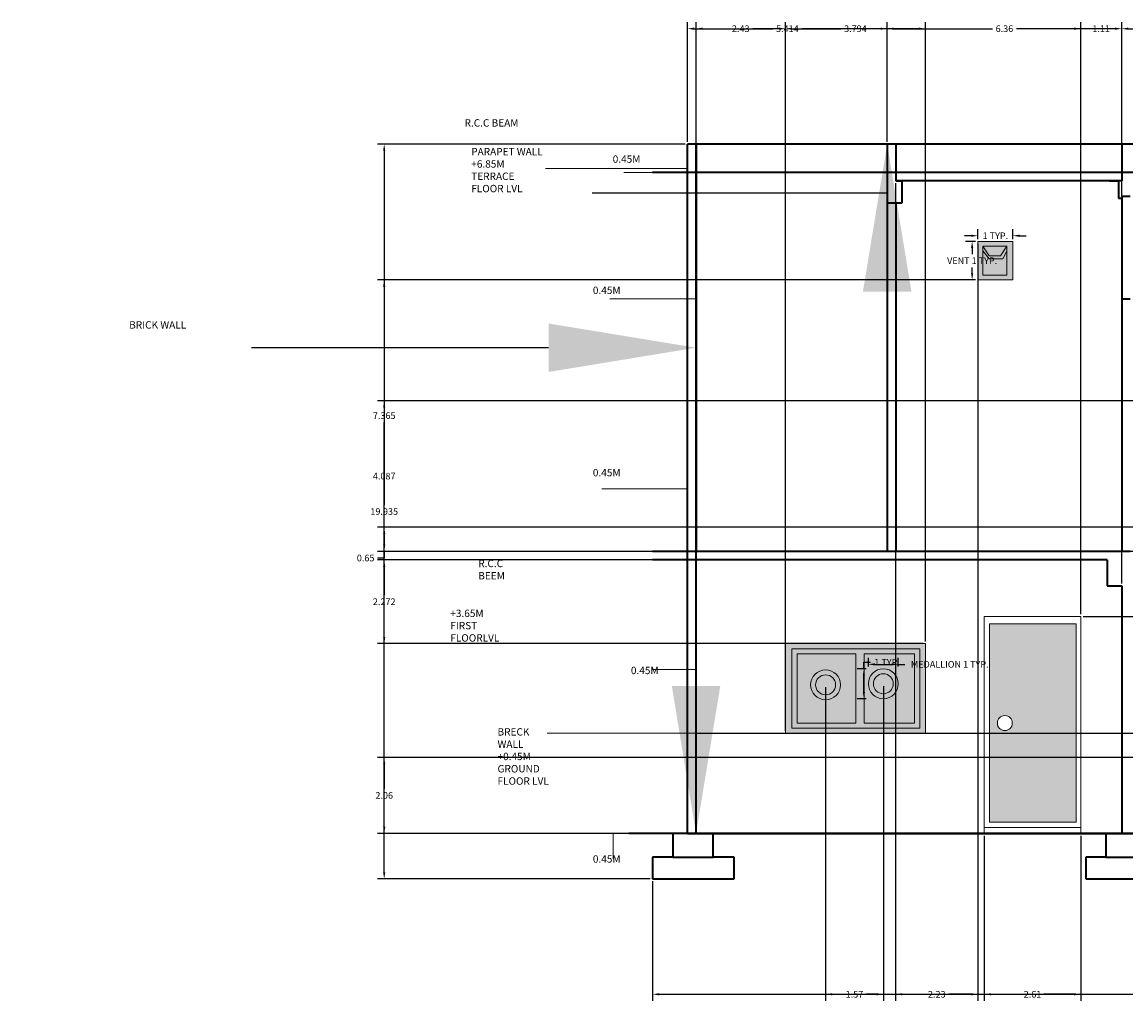
# Model space of a CAD drawing. Units: metres. Extents: x 1976.6 to 2045, y 823.7 to 850.3.
# Tile 1 of 3: x 1976.6 to 2006.5, y 823.7 to 850.3. Entities that reach past the tile are written whole.
import ezdxf
from ezdxf import colors
from ezdxf.entities.mleader import LeaderData, LeaderLine
from ezdxf.math import Vec2, Vec3

# ---------------------------------------------------------------- set-up
doc = ezdxf.new("R2010")
doc.units = ezdxf.units.M
for name, color, linetype, lineweight in [('A-ANNO-DIMS', 2, 'Continuous', 18), ('A-ANNO-TEXT', 7, 'Continuous', 18), ('A-COLS', 1, 'Continuous', 35), ('A-DOOR', 3, 'Continuous', 18), ('A-FLOR', 7, 'Continuous', 35), ('A-GLAZ', 4, 'Continuous', 18), ('A-GLAZ-PATT', 8, 'Continuous', 13), ('A-ROOF', 7, 'Continuous', 35), ('A-WALL', 7, 'Continuous', 35), ('A-WALL-PRPT', 7, 'Continuous', 35), ('S-BEAM', 1, 'Continuous', 35), ('S-FNDN', 1, 'Continuous', 35)]:
    doc.layers.add(name, color=color, linetype=linetype, lineweight=lineweight)
doc.styles.get("Standard").update_dxf_attribs({"font": 'arial.ttf'})
doc.dimstyles.get("Standard").update_dxf_attribs({"dimtxt": 0.18, "dimasz": 0.18, "dimexe": 0.18, "dimexo": 0.0625, "dimgap": 0.09, "dimtad": 0, "dimtih": 1, "dimtoh": 1, "dimdec": 4, "dimzin": 0, "dimdsep": 46, "dimtxsty": 'Standard', "dimcen": 0.09, "dimadec": 0, "dimazin": 0, "dimtfac": 1, "dimtdec": 4, "dimtofl": 0, "dimtmove": 0, "dimatfit": 3, "dimfxl": 1, "dimtolj": 1, "dimtzin": 0, "dimarcsym": 0})

# ---------------------------------------------------------------- blocks, each defined once
blk = doc.blocks.new('WIN-VENT')
h = blk.add_hatch(color=256)
h.dxf.hatch_style = 1
h.paths.add_polyline_path([(0.783, 0.781), (0.783, 0.912), (0.616, 0.651), (0.305, 0.651), (0.133, 0.912), (0.133, 0.788), (0.305, 0.57), (0.677, 0.57)], flags=0)
h.paths.add_polyline_path([(0.95, 1.042), (0, 1.042), (0, 0), (0.95, 0)])
h.paths.add_polyline_path([(0.783, 0.912), (0.783, 0.125), (0.133, 0.125), (0.133, 0.912)], flags=16)
h.paths.add_polyline_path([(0.783, 0.781), (0.783, 0.912), (0.133, 0.912), (0.133, 0.788), (0.305, 0.57), (0.677, 0.57)], flags=0)
h = blk.add_hatch(color=256)
h.dxf.hatch_style = 1
h.paths.add_polyline_path([(0.783, 0.781), (0.783, 0.912), (0.616, 0.651), (0.305, 0.651), (0.133, 0.912), (0.133, 0.788), (0.305, 0.57), (0.677, 0.57)])
h = blk.add_hatch(color=256)
h.dxf.hatch_style = 1
h.paths.add_polyline_path([(0.133, 0.912), (0.305, 0.651), (0.616, 0.651), (0.783, 0.912)])
h.paths.add_polyline_path([(0.783, 0.125), (0.783, 0.781), (0.677, 0.57), (0.305, 0.57), (0.133, 0.788), (0.133, 0.125)])
for p, q in [((0.133, 0.912), (0.305, 0.651)), ((0.133, 0.912), (0.133, 0.788)), ((0.616, 0.651), (0.783, 0.912)), ((0.133, 0.788), (0.305, 0.57)), ((0.305, 0.651), (0.616, 0.651)), ((0.677, 0.57), (0.783, 0.781)), ((0.305, 0.57), (0.677, 0.57))]:
    blk.add_line(p, q)
for points in [[(0, 1.042), (0.95, 1.042), (0.95, 0), (0, 0)], [(0.133, 0.912), (0.783, 0.912), (0.783, 0.125), (0.133, 0.125)]]:
    blk.add_lwpolyline(points, close=True)
blk = doc.blocks.new('FNDN-STEPPED-PAD')
for p, q in [((0.547, 1.235), (0.547, 0.59)), ((1.641, 0.59), (1.641, 1.235)), ((0.547, 0.59), (0, 0.59)), ((0, 0.59), (0, 0)), ((0.547, 0.59), (1.641, 0.59)), ((2.209, 0.59), (1.641, 0.59)), ((2.209, 0), (2.209, 0.59)), ((0, 0), (2.209, 0))]:
    blk.add_line(p, q)
blk = doc.blocks.new('DOOR-SINGLE-LEAF')
h = blk.add_hatch(color=256)
h.dxf.hatch_style = 1
h.paths.add_polyline_path([(2.349, 5.38), (2.224, 5.38), (0, 5.38), (0, 0), (2.349, 0)])
h.paths.add_polyline_path([(0.213, 2.69, -1), (0.619, 2.69, -1)], flags=16)
for p, q in [((2.349, 5.38), (2.224, 5.38)), ((2.224, 5.38), (2.349, 5.38)), ((2.349, 5.38), (2.349, 0)), ((2.349, 0), (0, 0))]:
    blk.add_line(p, q)
blk.add_lwpolyline([(0, 0), (0, 5.38), (2.349, 5.38)])
blk.add_circle((0.416, 2.69), 0.203)
blk = doc.blocks.new('WIN-RING-MEDALLION')
h = blk.add_hatch(color=256)
h.dxf.hatch_style = 1
h.paths.add_polyline_path([(-0.406, 0, 1), (0.406, 0, 1)])
h.paths.add_polyline_path([(0.271, 0, -1), (-0.271, 0, -1)], flags=16)
for radius in [0.406, 0.271]:
    blk.add_circle((0, 0), radius)
blk = doc.blocks.new('*D10')
at = {"layer": 'A-ANNO-DIMS', "color": 0, "lineweight": -2, "transparency": 16777216}
for p, q in [((2002.456, 844.342), (2002.182, 844.342)), ((2002.362, 844.162), (2002.362, 844.001)), ((2002.362, 843.48), (2002.362, 843.64)), ((2002.456, 843.3), (2002.182, 843.3))]:
    blk.add_line(p, q, dxfattribs=at)
at = {"layer": 'A-ANNO-DIMS', "color": 0, "transparency": 16777216}
for points in [[(2002.332, 844.162), (2002.392, 844.162), (2002.362, 844.342)], [(2002.332, 843.48), (2002.392, 843.48), (2002.362, 843.3)]]:
    blk.add_solid(points, dxfattribs=at)
at = {"layer": 'Defpoints', "color": 0, "transparency": 16777216}
for p in [(2002.362, 844.342), (2002.518, 844.342), (2002.518, 843.3)]:
    blk.add_point(p, dxfattribs=at)
at = {"layer": 'A-ANNO-DIMS', "color": 0, "transparency": 16777216, "insert": (2002.362, 843.821), "char_height": 0.18, "attachment_point": 5}
blk.add_mtext('\\A1;VENT 1 TYP.', dxfattribs=at)
blk = doc.blocks.new('*D11')
at = {"layer": 'A-ANNO-DIMS', "color": 0, "lineweight": -2, "transparency": 16777216}
for p, q in [((2002.518, 844.404), (2002.518, 844.678)), ((2003.468, 844.404), (2003.468, 844.678)), ((2002.338, 844.498), (2002.158, 844.498)), ((2003.648, 844.498), (2003.828, 844.498))]:
    blk.add_line(p, q, dxfattribs=at)
at = {"layer": 'A-ANNO-DIMS', "color": 0, "transparency": 16777216}
for points in [[(2002.338, 844.528), (2002.338, 844.468), (2002.518, 844.498)], [(2003.648, 844.528), (2003.648, 844.468), (2003.468, 844.498)]]:
    blk.add_solid(points, dxfattribs=at)
at = {"layer": 'Defpoints', "color": 0, "transparency": 16777216}
for p in [(2002.518, 844.342), (2003.468, 844.498), (2003.468, 844.342)]:
    blk.add_point(p, dxfattribs=at)
at = {"layer": 'A-ANNO-DIMS', "color": 0, "transparency": 16777216, "insert": (2002.993, 844.498), "char_height": 0.18, "attachment_point": 5}
blk.add_mtext('\\A1;1 TYP.', dxfattribs=at)
blk = doc.blocks.new('*D14')
at = {"layer": 'A-ANNO-DIMS', "color": 0, "lineweight": -2, "transparency": 16777216}
for p, q in [((1999.548, 832.812), (1999.548, 833.051)), ((1999.728, 832.871), (2000.179, 832.871)), ((2000.359, 832.812), (2000.359, 833.051)), ((2000.359, 832.871), (2000.539, 832.871))]:
    blk.add_line(p, q, dxfattribs=at)
at = {"layer": 'A-ANNO-DIMS', "color": 0, "transparency": 16777216}
for points in [[(1999.728, 832.901), (1999.728, 832.841), (1999.548, 832.871)], [(2000.179, 832.901), (2000.179, 832.841), (2000.359, 832.871)]]:
    blk.add_solid(points, dxfattribs=at)
at = {"layer": 'Defpoints', "color": 0, "transparency": 16777216}
for p in [(2000.359, 832.871), (1999.548, 832.75), (2000.359, 832.75)]:
    blk.add_point(p, dxfattribs=at)
at = {"layer": 'A-ANNO-DIMS', "color": 0, "transparency": 16777216, "insert": (2001.755, 832.871), "char_height": 0.18, "attachment_point": 5}
blk.add_mtext('\\A1;MEDALLION 1 TYP.', dxfattribs=at)
blk = doc.blocks.new('*D15')
at = {"layer": 'A-ANNO-DIMS', "color": 0, "lineweight": -2, "transparency": 16777216}
for p, q in [((1999.426, 832.75), (1999.426, 832.93)), ((1999.426, 832.93), (1999.606, 832.93)), ((1999.486, 832.75), (1999.246, 832.75)), ((1999.426, 832.119), (1999.426, 832.57)), ((1999.486, 831.939), (1999.246, 831.939))]:
    blk.add_line(p, q, dxfattribs=at)
at = {"layer": 'A-ANNO-DIMS', "color": 0, "transparency": 16777216}
for points in [[(1999.396, 832.57), (1999.456, 832.57), (1999.426, 832.75)], [(1999.396, 832.119), (1999.456, 832.119), (1999.426, 831.939)]]:
    blk.add_solid(points, dxfattribs=at)
at = {"layer": 'Defpoints', "color": 0, "transparency": 16777216}
for p in [(1999.426, 832.75), (1999.548, 832.75), (1999.548, 831.939)]:
    blk.add_point(p, dxfattribs=at)
at = {"layer": 'A-ANNO-DIMS', "color": 0, "transparency": 16777216, "insert": (2000.056, 832.93), "char_height": 0.18, "attachment_point": 5}
blk.add_mtext('\\A1;1 TYP.', dxfattribs=at)
blk = doc.blocks.new('*D16')
at = {"layer": 'A-ANNO-DIMS', "color": 0, "lineweight": -2, "transparency": 16777216}
for p, q in [((1993.695, 826.987), (1993.695, 823.74)), ((2041.154, 826.987), (2041.154, 823.74)), ((1993.875, 823.92), (2017.027, 823.92)), ((2040.974, 823.92), (2017.822, 823.92))]:
    blk.add_line(p, q, dxfattribs=at)
at = {"layer": 'A-ANNO-DIMS', "color": 0, "transparency": 16777216}
for points in [[(1993.875, 823.95), (1993.875, 823.89), (1993.695, 823.92)], [(2040.974, 823.95), (2040.974, 823.89), (2041.154, 823.92)]]:
    blk.add_solid(points, dxfattribs=at)
at = {"layer": 'Defpoints', "color": 0, "transparency": 16777216}
for p in [(1993.695, 827.05), (2041.154, 827.05), (2041.154, 823.92)]:
    blk.add_point(p, dxfattribs=at)
at = {"layer": 'A-ANNO-DIMS', "color": 0, "transparency": 16777216, "insert": (2017.425, 823.92), "char_height": 0.18, "attachment_point": 5}
blk.add_mtext('\\A1;47.46', dxfattribs=at)
blk = doc.blocks.new('*D17')
at = {"layer": 'A-ANNO-DIMS', "color": 0, "lineweight": -2, "transparency": 16777216}
for p, q in [((1994.582, 846.985), (1986.237, 846.985)), ((1986.417, 846.805), (1986.417, 837.199)), ((1986.417, 827.23), (1986.417, 836.835)), ((1993.633, 827.05), (1986.237, 827.05))]:
    blk.add_line(p, q, dxfattribs=at)
at = {"layer": 'A-ANNO-DIMS', "color": 0, "transparency": 16777216}
for points in [[(1986.387, 846.805), (1986.447, 846.805), (1986.417, 846.985)], [(1986.387, 827.23), (1986.447, 827.23), (1986.417, 827.05)]]:
    blk.add_solid(points, dxfattribs=at)
at = {"layer": 'Defpoints', "color": 0, "transparency": 16777216}
for p in [(1986.417, 846.985), (1994.645, 846.985), (1993.695, 827.05)]:
    blk.add_point(p, dxfattribs=at)
at = {"layer": 'A-ANNO-DIMS', "color": 0, "transparency": 16777216, "insert": (1986.417, 837.017), "char_height": 0.18, "attachment_point": 5}
blk.add_mtext('\\A1;19.935', dxfattribs=at)
blk = doc.blocks.new('*D18')
at = {"layer": 'A-ANNO-DIMS', "color": 0, "lineweight": -2, "transparency": 16777216}
for p, q in [((1994.645, 847.047), (1994.645, 850.295)), ((2000.058, 847.047), (2000.058, 850.295)), ((1994.825, 850.115), (1996.958, 850.115)), ((1999.878, 850.115), (1997.745, 850.115))]:
    blk.add_line(p, q, dxfattribs=at)
at = {"layer": 'A-ANNO-DIMS', "color": 0, "transparency": 16777216}
for points in [[(1994.825, 850.145), (1994.825, 850.085), (1994.645, 850.115)], [(1999.878, 850.145), (1999.878, 850.085), (2000.058, 850.115)]]:
    blk.add_solid(points, dxfattribs=at)
at = {"layer": 'Defpoints', "color": 0, "transparency": 16777216}
for p in [(2000.058, 850.115), (1994.645, 846.985), (2000.058, 846.985)]:
    blk.add_point(p, dxfattribs=at)
at = {"layer": 'A-ANNO-DIMS', "color": 0, "transparency": 16777216, "insert": (1997.351, 850.115), "char_height": 0.18, "attachment_point": 5}
blk.add_mtext('\\A1;5.414', dxfattribs=at)
blk = doc.blocks.new('*D19')
at = {"layer": 'A-ANNO-DIMS', "color": 0, "lineweight": -2, "transparency": 16777216}
for p, q in [((2000.058, 847.047), (2000.058, 850.295)), ((2006.418, 847.047), (2006.418, 850.295)), ((2000.238, 850.115), (2002.914, 850.115)), ((2006.238, 850.115), (2003.562, 850.115))]:
    blk.add_line(p, q, dxfattribs=at)
at = {"layer": 'A-ANNO-DIMS', "color": 0, "transparency": 16777216}
for points in [[(2000.238, 850.145), (2000.238, 850.085), (2000.058, 850.115)], [(2006.238, 850.145), (2006.238, 850.085), (2006.418, 850.115)]]:
    blk.add_solid(points, dxfattribs=at)
at = {"layer": 'Defpoints', "color": 0, "transparency": 16777216}
for p in [(2006.418, 850.115), (2000.058, 846.985), (2006.418, 846.985)]:
    blk.add_point(p, dxfattribs=at)
at = {"layer": 'A-ANNO-DIMS', "color": 0, "transparency": 16777216, "insert": (2003.238, 850.115), "char_height": 0.18, "attachment_point": 5}
blk.add_mtext('\\A1;6.36', dxfattribs=at)
blk = doc.blocks.new('*D20')
at = {"layer": 'A-ANNO-DIMS', "color": 0, "lineweight": -2, "transparency": 16777216}
for p, q in [((2006.418, 847.047), (2006.418, 850.295)), ((2019.995, 847.047), (2019.995, 850.295)), ((2006.598, 850.115), (2012.751, 850.115)), ((2019.815, 850.115), (2013.661, 850.115))]:
    blk.add_line(p, q, dxfattribs=at)
at = {"layer": 'A-ANNO-DIMS', "color": 0, "transparency": 16777216}
for points in [[(2006.598, 850.145), (2006.598, 850.085), (2006.418, 850.115)], [(2019.815, 850.145), (2019.815, 850.085), (2019.995, 850.115)]]:
    blk.add_solid(points, dxfattribs=at)
at = {"layer": 'Defpoints', "color": 0, "transparency": 16777216}
for p in [(2019.995, 850.115), (2006.418, 846.985), (2019.995, 846.985)]:
    blk.add_point(p, dxfattribs=at)
at = {"layer": 'A-ANNO-DIMS', "color": 0, "transparency": 16777216, "insert": (2013.206, 850.115), "char_height": 0.18, "attachment_point": 5}
blk.add_mtext('\\A1;13.577', dxfattribs=at)
blk = doc.blocks.new('*D31')
at = {"layer": 'A-ANNO-DIMS', "color": 0, "lineweight": -2, "transparency": 16777216}
for p, q in [((1994.875, 828.347), (1994.875, 850.295)), ((1997.3, 831.068), (1997.3, 850.295)), ((1995.055, 850.115), (1995.762, 850.115)), ((1997.12, 850.115), (1996.413, 850.115))]:
    blk.add_line(p, q, dxfattribs=at)
at = {"layer": 'A-ANNO-DIMS', "color": 0, "transparency": 16777216}
for points in [[(1995.055, 850.145), (1995.055, 850.085), (1994.875, 850.115)], [(1997.12, 850.145), (1997.12, 850.085), (1997.3, 850.115)]]:
    blk.add_solid(points, dxfattribs=at)
at = {"layer": 'Defpoints', "color": 0, "transparency": 16777216}
for p in [(1997.3, 850.115), (1997.3, 831.006), (1994.875, 828.285)]:
    blk.add_point(p, dxfattribs=at)
at = {"layer": 'A-ANNO-DIMS', "color": 0, "transparency": 16777216, "insert": (1996.087, 850.115), "char_height": 0.18, "attachment_point": 5}
blk.add_mtext('\\A1;2.43', dxfattribs=at)
blk = doc.blocks.new('*D32')
at = {"layer": 'A-ANNO-DIMS', "color": 0, "lineweight": -2, "transparency": 16777216}
for p, q in [((1997.363, 831.006), (2044.464, 831.006)), ((2044.284, 830.826), (2044.284, 829.826)), ((2044.284, 828.465), (2044.284, 829.465)), ((1994.937, 828.285), (2044.464, 828.285))]:
    blk.add_line(p, q, dxfattribs=at)
at = {"layer": 'A-ANNO-DIMS', "color": 0, "transparency": 16777216}
for points in [[(2044.254, 830.826), (2044.314, 830.826), (2044.284, 831.006)], [(2044.254, 828.465), (2044.314, 828.465), (2044.284, 828.285)]]:
    blk.add_solid(points, dxfattribs=at)
at = {"layer": 'Defpoints', "color": 0, "transparency": 16777216}
for p in [(1997.3, 831.006), (1994.875, 828.285), (2044.284, 828.285)]:
    blk.add_point(p, dxfattribs=at)
at = {"layer": 'A-ANNO-DIMS', "color": 0, "transparency": 16777216, "insert": (2044.284, 829.645), "char_height": 0.18, "attachment_point": 5}
blk.add_mtext('\\A1;2.721', dxfattribs=at)
blk = doc.blocks.new('*D33')
at = {"layer": 'A-ANNO-DIMS', "color": 0, "lineweight": -2, "transparency": 16777216}
for p, q in [((1997.3, 833.495), (1997.3, 850.295)), ((2001.094, 833.495), (2001.094, 850.295)), ((1997.48, 850.115), (1998.804, 850.115)), ((2000.914, 850.115), (1999.59, 850.115))]:
    blk.add_line(p, q, dxfattribs=at)
at = {"layer": 'A-ANNO-DIMS', "color": 0, "transparency": 16777216}
for points in [[(1997.48, 850.145), (1997.48, 850.085), (1997.3, 850.115)], [(2000.914, 850.145), (2000.914, 850.085), (2001.094, 850.115)]]:
    blk.add_solid(points, dxfattribs=at)
at = {"layer": 'Defpoints', "color": 0, "transparency": 16777216}
for p in [(2001.094, 850.115), (1997.3, 833.433), (2001.094, 833.433)]:
    blk.add_point(p, dxfattribs=at)
at = {"layer": 'A-ANNO-DIMS', "color": 0, "transparency": 16777216, "insert": (1999.197, 850.115), "char_height": 0.18, "attachment_point": 5}
blk.add_mtext('\\A1;3.794', dxfattribs=at)
blk = doc.blocks.new('*D34')
at = {"layer": 'A-ANNO-DIMS', "color": 0, "lineweight": -2, "transparency": 16777216}
for p, q in [((2005.961, 835.705), (1986.237, 835.705)), ((1986.417, 835.525), (1986.417, 834.749)), ((1986.417, 833.613), (1986.417, 834.389)), ((2001.032, 833.433), (1986.237, 833.433))]:
    blk.add_line(p, q, dxfattribs=at)
at = {"layer": 'A-ANNO-DIMS', "color": 0, "transparency": 16777216}
for points in [[(1986.387, 835.525), (1986.447, 835.525), (1986.417, 835.705)], [(1986.387, 833.613), (1986.447, 833.613), (1986.417, 833.433)]]:
    blk.add_solid(points, dxfattribs=at)
at = {"layer": 'Defpoints', "color": 0, "transparency": 16777216}
for p in [(1986.417, 835.705), (2006.024, 835.705), (2001.094, 833.433)]:
    blk.add_point(p, dxfattribs=at)
at = {"layer": 'A-ANNO-DIMS', "color": 0, "transparency": 16777216, "insert": (1986.417, 834.569), "char_height": 0.18, "attachment_point": 5}
blk.add_mtext('\\A1;2.272', dxfattribs=at)
blk = doc.blocks.new('*D35')
at = {"layer": 'A-ANNO-DIMS', "color": 0, "lineweight": -2, "transparency": 16777216}
for p, q in [((1998.388, 832.253), (1998.388, 823.74)), ((1999.954, 832.282), (1999.954, 823.74)), ((1998.568, 823.92), (1998.856, 823.92)), ((1999.774, 823.92), (1999.486, 823.92))]:
    blk.add_line(p, q, dxfattribs=at)
at = {"layer": 'A-ANNO-DIMS', "color": 0, "transparency": 16777216}
for points in [[(1998.568, 823.95), (1998.568, 823.89), (1998.388, 823.92)], [(1999.774, 823.95), (1999.774, 823.89), (1999.954, 823.92)]]:
    blk.add_solid(points, dxfattribs=at)
at = {"layer": 'Defpoints', "color": 0, "transparency": 16777216}
for p in [(1998.388, 832.315), (1999.954, 832.344), (1999.954, 823.92)]:
    blk.add_point(p, dxfattribs=at)
at = {"layer": 'A-ANNO-DIMS', "color": 0, "transparency": 16777216, "insert": (1999.171, 823.92), "char_height": 0.18, "attachment_point": 5}
blk.add_mtext('\\A1;1.57', dxfattribs=at)
blk = doc.blocks.new('*D36')
at = {"layer": 'A-ANNO-DIMS', "color": 0, "lineweight": -2, "transparency": 16777216}
for p, q in [((2005.307, 834.228), (2005.307, 850.295)), ((2006.418, 835.06), (2006.418, 850.295)), ((2005.127, 850.115), (2004.947, 850.115)), ((2006.598, 850.115), (2006.778, 850.115))]:
    blk.add_line(p, q, dxfattribs=at)
at = {"layer": 'A-ANNO-DIMS', "color": 0, "transparency": 16777216}
for points in [[(2005.127, 850.145), (2005.127, 850.085), (2005.307, 850.115)], [(2006.598, 850.145), (2006.598, 850.085), (2006.418, 850.115)]]:
    blk.add_solid(points, dxfattribs=at)
at = {"layer": 'Defpoints', "color": 0, "transparency": 16777216}
for p in [(2006.418, 850.115), (2006.418, 834.998), (2005.307, 834.166)]:
    blk.add_point(p, dxfattribs=at)
at = {"layer": 'A-ANNO-DIMS', "color": 0, "transparency": 16777216, "insert": (2005.862, 850.115), "char_height": 0.18, "attachment_point": 5}
blk.add_mtext('\\A1;1.11', dxfattribs=at)
blk = doc.blocks.new('*D37')
at = {"layer": 'A-ANNO-DIMS', "color": 0, "lineweight": -2, "transparency": 16777216}
for p, q in [((2002.692, 828.222), (2002.692, 823.74)), ((2005.307, 828.222), (2005.307, 823.74)), ((2002.872, 823.92), (2003.692, 823.92)), ((2005.127, 823.92), (2004.307, 823.92))]:
    blk.add_line(p, q, dxfattribs=at)
at = {"layer": 'A-ANNO-DIMS', "color": 0, "transparency": 16777216}
for points in [[(2002.872, 823.95), (2002.872, 823.89), (2002.692, 823.92)], [(2005.127, 823.95), (2005.127, 823.89), (2005.307, 823.92)]]:
    blk.add_solid(points, dxfattribs=at)
at = {"layer": 'Defpoints', "color": 0, "transparency": 16777216}
for p in [(2002.692, 828.285), (2005.307, 828.285), (2005.307, 823.92)]:
    blk.add_point(p, dxfattribs=at)
at = {"layer": 'A-ANNO-DIMS', "color": 0, "transparency": 16777216, "insert": (2004, 823.92), "char_height": 0.18, "attachment_point": 5}
blk.add_mtext('\\A1;2.61', dxfattribs=at)
blk = doc.blocks.new('*D38')
at = {"layer": 'A-ANNO-DIMS', "color": 0, "lineweight": -2, "transparency": 16777216}
for p, q in [((2005.369, 834.166), (2044.464, 834.166)), ((2044.284, 833.986), (2044.284, 831.407)), ((2044.284, 828.465), (2044.284, 831.043)), ((2005.369, 828.285), (2044.464, 828.285))]:
    blk.add_line(p, q, dxfattribs=at)
at = {"layer": 'A-ANNO-DIMS', "color": 0, "transparency": 16777216}
for points in [[(2044.254, 833.986), (2044.314, 833.986), (2044.284, 834.166)], [(2044.254, 828.465), (2044.314, 828.465), (2044.284, 828.285)]]:
    blk.add_solid(points, dxfattribs=at)
at = {"layer": 'Defpoints', "color": 0, "transparency": 16777216}
for p in [(2005.307, 834.166), (2005.307, 828.285), (2044.284, 828.285)]:
    blk.add_point(p, dxfattribs=at)
at = {"layer": 'A-ANNO-DIMS', "color": 0, "transparency": 16777216, "insert": (2044.284, 831.225), "char_height": 0.18, "attachment_point": 5}
blk.add_mtext('\\A1;5.881', dxfattribs=at)
blk = doc.blocks.new('*D41')
at = {"layer": 'A-ANNO-DIMS', "color": 0, "lineweight": -2, "transparency": 16777216}
for p, q in [((2026.178, 830.345), (1986.237, 830.345)), ((1986.417, 830.165), (1986.417, 829.497)), ((1986.417, 828.465), (1986.417, 829.133)), ((2025.843, 828.285), (1986.237, 828.285))]:
    blk.add_line(p, q, dxfattribs=at)
at = {"layer": 'A-ANNO-DIMS', "color": 0, "transparency": 16777216}
for points in [[(1986.387, 830.165), (1986.447, 830.165), (1986.417, 830.345)], [(1986.387, 828.465), (1986.447, 828.465), (1986.417, 828.285)]]:
    blk.add_solid(points, dxfattribs=at)
at = {"layer": 'Defpoints', "color": 0, "transparency": 16777216}
for p in [(2026.24, 830.345), (1986.417, 828.285), (2025.906, 828.285)]:
    blk.add_point(p, dxfattribs=at)
at = {"layer": 'A-ANNO-DIMS', "color": 0, "transparency": 16777216, "insert": (1986.417, 829.315), "char_height": 0.18, "attachment_point": 5}
blk.add_mtext('\\A1;2.06', dxfattribs=at)
blk = doc.blocks.new('*D42')
at = {"layer": 'A-ANNO-DIMS', "color": 0, "lineweight": -2, "transparency": 16777216}
for p, q in [((2021.404, 840.022), (1986.237, 840.022)), ((1986.417, 839.842), (1986.417, 838.16)), ((1986.417, 836.115), (1986.417, 837.796)), ((2020.162, 835.935), (1986.237, 835.935))]:
    blk.add_line(p, q, dxfattribs=at)
at = {"layer": 'A-ANNO-DIMS', "color": 0, "transparency": 16777216}
for points in [[(1986.387, 839.842), (1986.447, 839.842), (1986.417, 840.022)], [(1986.387, 836.115), (1986.447, 836.115), (1986.417, 835.935)]]:
    blk.add_solid(points, dxfattribs=at)
at = {"layer": 'Defpoints', "color": 0, "transparency": 16777216}
for p in [(2021.467, 840.022), (1986.417, 835.935), (2020.225, 835.935)]:
    blk.add_point(p, dxfattribs=at)
at = {"layer": 'A-ANNO-DIMS', "color": 0, "transparency": 16777216, "insert": (1986.417, 837.978), "char_height": 0.18, "attachment_point": 5}
blk.add_mtext('\\A1;4.087', dxfattribs=at)
blk = doc.blocks.new('*D44')
at = {"layer": 'A-ANNO-DIMS', "color": 0, "lineweight": -2, "transparency": 16777216}
for p, q in [((2000.288, 845.922), (2000.288, 823.74)), ((2002.518, 844.279), (2002.518, 823.74)), ((2000.468, 823.92), (2001.078, 823.92)), ((2002.338, 823.92), (2001.729, 823.92))]:
    blk.add_line(p, q, dxfattribs=at)
at = {"layer": 'A-ANNO-DIMS', "color": 0, "transparency": 16777216}
for points in [[(2000.468, 823.95), (2000.468, 823.89), (2000.288, 823.92)], [(2002.338, 823.95), (2002.338, 823.89), (2002.518, 823.92)]]:
    blk.add_solid(points, dxfattribs=at)
at = {"layer": 'Defpoints', "color": 0, "transparency": 16777216}
for p in [(2000.288, 845.985), (2002.518, 844.342), (2002.518, 823.92)]:
    blk.add_point(p, dxfattribs=at)
at = {"layer": 'A-ANNO-DIMS', "color": 0, "transparency": 16777216, "insert": (2001.403, 823.92), "char_height": 0.18, "attachment_point": 5}
blk.add_mtext('\\A1;2.23', dxfattribs=at)
blk = doc.blocks.new('*D45')
at = {"layer": 'A-ANNO-DIMS', "color": 0, "lineweight": -2, "transparency": 16777216}
for p, q in [((2002.456, 843.3), (1986.237, 843.3)), ((1986.417, 843.12), (1986.417, 839.799)), ((1986.417, 836.115), (1986.417, 839.435)), ((2000.226, 835.935), (1986.237, 835.935))]:
    blk.add_line(p, q, dxfattribs=at)
at = {"layer": 'A-ANNO-DIMS', "color": 0, "transparency": 16777216}
for points in [[(1986.387, 843.12), (1986.447, 843.12), (1986.417, 843.3)], [(1986.387, 836.115), (1986.447, 836.115), (1986.417, 835.935)]]:
    blk.add_solid(points, dxfattribs=at)
at = {"layer": 'Defpoints', "color": 0, "transparency": 16777216}
for p in [(1986.417, 843.3), (2002.518, 843.3), (2000.288, 835.935)]:
    blk.add_point(p, dxfattribs=at)
at = {"layer": 'A-ANNO-DIMS', "color": 0, "transparency": 16777216, "insert": (1986.417, 839.617), "char_height": 0.18, "attachment_point": 5}
blk.add_mtext('\\A1;7.365', dxfattribs=at)
blk = doc.blocks.new('*D48')
at = {"layer": 'A-ANNO-DIMS', "color": 0, "lineweight": -2, "transparency": 16777216}
for p, q in [((2038.162, 836.589), (1986.237, 836.589)), ((1986.417, 836.409), (1986.417, 836.115)), ((2039.726, 835.935), (1986.237, 835.935)), ((1986.417, 835.935), (1986.417, 835.755)), ((1986.417, 835.755), (1986.237, 835.755))]:
    blk.add_line(p, q, dxfattribs=at)
at = {"layer": 'A-ANNO-DIMS', "color": 0, "transparency": 16777216}
for points in [[(1986.387, 836.409), (1986.447, 836.409), (1986.417, 836.589)], [(1986.387, 836.115), (1986.447, 836.115), (1986.417, 835.935)]]:
    blk.add_solid(points, dxfattribs=at)
at = {"layer": 'Defpoints', "color": 0, "transparency": 16777216}
for p in [(2038.224, 836.589), (1986.417, 835.935), (2039.788, 835.935)]:
    blk.add_point(p, dxfattribs=at)
at = {"layer": 'A-ANNO-DIMS', "color": 0, "transparency": 16777216, "insert": (1985.913, 835.755), "char_height": 0.18, "attachment_point": 5}
blk.add_mtext('\\A1;0.65', dxfattribs=at)

msp = doc.modelspace()

# ---------------------------------------------------------------- hatches: boundary and pattern name
at = {"layer": 'A-GLAZ-PATT'}
h = msp.add_hatch(color=256, dxfattribs=at)
h.dxf.hatch_style = 1
h.paths.add_polyline_path([(2001.0942, 833.433), (1997.3001, 833.433), (1997.3001, 831.0057), (2001.0942, 831.0057)])
h.paths.add_polyline_path([(2000.9464, 833.2948), (2000.9464, 831.1409), (1997.4738, 831.1409), (1997.4738, 833.2948)], flags=16)
h.paths.add_polyline_path([(2000.7947, 833.1536), (2000.7947, 831.2759), (1999.435, 831.2759), (1999.435, 833.1536)], flags=0)
h.paths.add_polyline_path([(1999.205, 833.1536), (1999.205, 831.2759), (1997.6153, 831.2759), (1997.6153, 833.1536)], flags=0)
h = msp.add_hatch(color=256, dxfattribs=at)
h.dxf.hatch_style = 1
h.paths.add_polyline_path([(2000.9464, 833.2948), (1997.4738, 833.2948), (1997.4738, 831.1409), (2000.9464, 831.1409)])
h.paths.add_polyline_path([(1999.435, 833.1536), (2000.7947, 833.1536), (2000.7947, 831.2759), (1999.435, 831.2759)], flags=16)
h.paths.add_polyline_path([(1999.205, 831.2759), (1997.6153, 831.2759), (1997.6153, 833.1536), (1999.205, 833.1536)], flags=16)
h = msp.add_hatch(color=256, dxfattribs=at)
h.dxf.hatch_style = 1
h.paths.add_polyline_path([(2000.7947, 833.1536), (1999.435, 833.1536), (1999.435, 831.2759), (2000.7947, 831.2759)])
h.paths.add_polyline_path([(1999.205, 833.1536), (1997.6153, 833.1536), (1997.6153, 831.2759), (1999.205, 831.2759)])

# ---------------------------------------------------------------- linework, layer by layer
at = {"layer": 'A-ANNO-DIMS'}
for p, q in [((1993.6952, 846.2148), (1992.9202, 846.2148)), ((1993.6952, 842.7848), (1992.5404, 842.7848)), ((1994.8746, 842.7848), (1993.6952, 842.7848)), ((1994.6446, 837.6348), (1992.3182, 837.6348)), ((1994.8746, 832.7348), (1993.6952, 832.7348)), ((1993.0497, 828.2848), (1992.6275, 828.2848)), ((1992.6275, 828.2848), (1992.6275, 827.6049))]:
    msp.add_line(p, q, dxfattribs=at)
at = {"layer": 'A-ANNO-TEXT'}
for p, q in [((1994.6446, 846.9848), (1994.6446, 846.5098)), ((1994.6446, 846.5098), (1994.6446, 846.3224)), ((1994.6446, 846.3224), (1990.7874, 846.3224)), ((1993.6952, 835.7048), (1989.5474, 835.7048)), ((1994.8746, 831.0057), (1990.8363, 831.0057))]:
    msp.add_line(p, q, dxfattribs=at)
at = {"layer": 'A-COLS'}
for p, q in [((2006.4179, 846.9848), (2006.4179, 845.9848)), ((2006.4179, 845.5737), (2006.4179, 835.9348)), ((2006.4179, 842.7848), (2006.6479, 842.7848)), ((2006.4179, 834.9975), (2006.4179, 828.2848))]:
    msp.add_line(p, q, dxfattribs=at)
at = {"layer": 'A-DOOR'}
for p, q in [((2002.6924, 834.1656), (2002.6924, 828.2848)), ((2005.3067, 834.1656), (2002.6924, 834.1656)), ((2005.3067, 828.2848), (2005.3067, 834.1656)), ((2002.6924, 828.2848), (2002.6924, 828.4471)), ((2002.6924, 828.4471), (2005.3067, 828.4471)), ((2002.6924, 828.2848), (2005.3067, 828.2848))]:
    msp.add_line(p, q, dxfattribs=at)
msp.add_lwpolyline([(2005.3067, 833.9675), (2005.3067, 828.2848), (2002.8326, 828.2848)], dxfattribs=at)
at = {"layer": 'A-FLOR'}
for p, q in [((2006.6479, 835.9348), (1993.6952, 835.9348)), ((2006.0238, 835.7048), (1993.6952, 835.7048)), ((2040.5852, 828.2848), (1993.0497, 828.2848)), ((2040.5852, 828.2848), (1994.6446, 828.2848)), ((1994.6446, 828.2848), (2009.2074, 828.2848))]:
    msp.add_line(p, q, dxfattribs=at)
at = {"layer": 'A-GLAZ'}
for p, q in [((1999.205, 833.1536), (1999.205, 831.2759)), ((1999.435, 833.1536), (1999.435, 831.2759))]:
    msp.add_line(p, q, dxfattribs=at)
for points in [[(1997.3001, 833.433), (2001.0942, 833.433), (2001.0942, 831.0057), (1997.3001, 831.0057)], [(1997.4738, 833.2948), (2000.9464, 833.2948), (2000.9464, 831.1409), (1997.4738, 831.1409)]]:
    msp.add_lwpolyline(points, close=True, dxfattribs=at)
for points in [[(1999.205, 831.2759), (1997.6153, 831.2759), (1997.6153, 833.1536), (1999.205, 833.1536)], [(1999.435, 833.1536), (2000.7947, 833.1536), (2000.7947, 831.2759), (1999.435, 831.2759)]]:
    msp.add_lwpolyline(points, dxfattribs=at)
at = {"layer": 'A-ROOF'}
for p, q in [((2040.0184, 846.2148), (1993.6952, 846.2148)), ((2006.4179, 845.9848), (2000.2883, 845.9848)), ((2006.4179, 845.9848), (2006.0884, 845.9848))]:
    msp.add_line(p, q, dxfattribs=at)
at = {"layer": 'A-WALL'}
for p, q in [((1994.6446, 828.2848), (1994.6446, 846.9848)), ((1994.8746, 828.2848), (1994.8746, 846.9848)), ((1994.8746, 846.9848), (1994.8746, 835.9348)), ((2000.0583, 846.9848), (2000.0583, 835.9348)), ((2000.2883, 846.9848), (2000.2883, 845.9848)), ((2000.2883, 845.3784), (2000.2883, 835.9348))]:
    msp.add_line(p, q, dxfattribs=at)
at = {"layer": 'A-WALL-PRPT'}
msp.add_line((2040.0184, 846.9848), (1994.6446, 846.9848), dxfattribs=at)
at = {"layer": 'S-BEAM'}
for p, q in [((2000.2883, 845.9848), (2000.4582, 845.9848)), ((2000.4582, 845.9848), (2000.4582, 845.3784)), ((2006.0884, 845.9848), (2006.3279, 845.9848)), ((2006.3279, 845.9848), (2006.3614, 845.9848)), ((2006.3279, 845.9848), (2006.3279, 845.5197)), ((2006.3279, 845.5197), (2006.4179, 845.5197)), ((2006.4179, 845.5737), (2006.6479, 845.5737)), ((2000.4582, 845.3784), (2000.0583, 845.3784)), ((2006.0238, 835.7048), (2006.0238, 834.9975)), ((2006.0238, 834.9975), (2006.4179, 834.9975))]:
    msp.add_line(p, q, dxfattribs=at)
at = {"layer": 'S-FNDN'}
msp.add_line((1994.6446, 828.2848), (1994.242, 828.2848), dxfattribs=at)

# ---------------------------------------------------------------- block references
at = {"layer": 'A-DOOR'}
msp.add_blockref('DOOR-SINGLE-LEAF', (2002.833, 828.587), dxfattribs=at)
at = {"layer": 'A-GLAZ'}
for name, p in [('WIN-VENT', (2002.518, 843.3)), ('WIN-RING-MEDALLION', (1998.3881, 832.3151)), ('WIN-RING-MEDALLION', (1999.9537, 832.3442))]:
    msp.add_blockref(name, p, dxfattribs=at)
at = {"layer": 'S-FNDN'}
for p in [(1993.695, 827.05), (2005.4419, 827.05)]:
    msp.add_blockref('FNDN-STEPPED-PAD', p, dxfattribs=at)

# ---------------------------------------------------------------- texts
at = {"layer": 'A-ANNO-DIMS', "char_height": 0.2, "attachment_point": 1}
for insert in [(1992.6139, 846.6782), (1992.0757, 843.1174), (1992.0757, 838.1716), (1993.1075, 832.8053), (1992.0757, 827.6912)]:
    msp.add_mtext_dynamic_manual_height_columns('0.45M', width=0.489427, gutter_width=12.5, heights=[0], dxfattribs=dict(at, insert=insert))
at = {"layer": 'A-ANNO-TEXT', "char_height": 0.2, "attachment_point": 1}
for s, width, insert in [('PARAPET WALL +6.85M TERRACE FLOOR LVL ', 2.009703, (1988.7777, 846.8785)), ('\\PBRICK WALL ', 3.243202, (1979.5006, 842.5127)), ('R.C.C BEEM', 0.636736, (1988.9675, 835.7071)), ('\\P\\P\\P\\P+3.65M FIRST FLOORLVL ', 1.338048, (1988.2094, 835.6879)), ('BRECK WALL +0.45M GROUND FLOOR LVL', 1.614838, (1989.4906, 831.1387))]:
    msp.add_mtext_dynamic_manual_height_columns(s, width=width, gutter_width=12.5, heights=[0], dxfattribs=dict(at, insert=insert))

# ---------------------------------------------------------------- dimensions: what is measured, and where the dimension line sits
at = {"layer": 'A-ANNO-DIMS'}
for base, p1, p2, override, picture, middle in [((2000.0583, 850.1148), (1994.6446, 846.9848), (2000.0583, 846.9848), {"dimdec": 3, "dimlfac": 1, "dimrnd": 0, "dimzin": 0, "dimdsep": 46, "dimlunit": 2}, '*D18', (1997.3514, 850.1148)), ((1997.3001, 850.1148), (1994.8746, 828.2848), (1997.3001, 831.0057), {"dimdec": 2, "dimlfac": 1, "dimrnd": 0, "dimzin": 0, "dimdsep": 46, "dimlunit": 2}, '*D31', (1996.0874, 850.1148)), ((2001.0942, 850.1148), (1997.3001, 833.433), (2001.0942, 833.433), {"dimdec": 3, "dimlfac": 1, "dimrnd": 0, "dimzin": 0, "dimdsep": 46, "dimlunit": 2}, '*D33', (1999.1971, 850.1148)), ((2006.4179, 850.1148), (2000.0583, 846.9848), (2006.4179, 846.9848), {"dimdec": 2, "dimlfac": 1, "dimrnd": 0, "dimzin": 0, "dimdsep": 46, "dimlunit": 2}, '*D19', (2003.2381, 850.1148)), ((2006.4179, 850.1148), (2005.3067, 834.1656), (2006.4179, 834.9975), {"dimdec": 2, "dimlfac": 1, "dimrnd": 0, "dimzin": 0, "dimdsep": 46, "dimlunit": 2}, '*D36', (2005.8623, 850.1148)), ((2019.9947, 850.1148), (2006.4179, 846.9848), (2019.9947, 846.9848), {"dimdec": 3, "dimlfac": 1, "dimrnd": 0, "dimzin": 0, "dimdsep": 46, "dimlunit": 2}, '*D20', (2013.2063, 850.1148)), ((2002.5181, 823.9197), (2000.2883, 845.9848), (2002.5181, 844.3417), {"dimdec": 2, "dimlfac": 1, "dimrnd": 0, "dimzin": 0, "dimdsep": 46, "dimlunit": 2}, '*D44', (2001.4032, 823.9197)), ((1999.9537, 823.9197), (1998.3881, 832.3151), (1999.9537, 832.3442), {"dimdec": 2, "dimlfac": 1, "dimrnd": 0, "dimzin": 0, "dimdsep": 46, "dimlunit": 2}, '*D35', (1999.1709, 823.9197)), ((2005.3067, 823.9197), (2002.6924, 828.2848), (2005.3067, 828.2848), {"dimdec": 2, "dimlfac": 1, "dimrnd": 0, "dimzin": 0, "dimdsep": 46, "dimlunit": 2}, '*D37', (2003.9995, 823.9197)), ((2041.1538, 823.9197), (1993.6952, 827.0497), (2041.1538, 827.0497), {"dimdec": 2, "dimlfac": 1, "dimrnd": 0, "dimzin": 0, "dimdsep": 46, "dimlunit": 2}, '*D16', (2017.4245, 823.9197))]:
    dim = msp.add_linear_dim(base=base, p1=p1, p2=p2, dimstyle='Standard', override=override, dxfattribs=at)
    dim.commit()
    dim.dimension.update_dxf_attribs({"geometry": picture, "text_midpoint": middle})
for base, p1, p2, override, picture, middle in [((1986.4174, 846.9848), (1993.6952, 827.0497), (1994.6446, 846.9848), {"dimdec": 3, "dimlfac": 1, "dimrnd": 0, "dimzin": 0, "dimdsep": 46, "dimlunit": 2}, '*D17', (1986.4174, 837.0173)), ((1986.4174, 843.2997), (2000.2883, 835.9348), (2002.5181, 843.2997), {"dimdec": 3, "dimlfac": 1, "dimrnd": 0, "dimzin": 0, "dimdsep": 46, "dimlunit": 2}, '*D45', (1986.4174, 839.6173)), ((1986.4174, 835.9348), (2021.4669, 840.0217), (2020.2247, 835.9348), {"dimdec": 3, "dimlfac": 1, "dimrnd": 0, "dimzin": 0, "dimdsep": 46, "dimlunit": 2}, '*D42', (1986.4174, 837.9782)), ((1986.4174, 835.9348), (2038.2243, 836.5887), (2039.7884, 835.9348), {"dimdec": 2, "dimlfac": 1, "dimrnd": 0, "dimzin": 0, "dimdsep": 46, "dimlunit": 2}, '*D48', (1985.913, 835.7548)), ((1986.4174, 835.7048), (2001.0942, 833.433), (2006.0238, 835.7048), {"dimdec": 3, "dimlfac": 1, "dimrnd": 0, "dimzin": 0, "dimdsep": 46, "dimlunit": 2}, '*D34', (1986.4174, 834.5689)), ((2044.2838, 828.2848), (2005.3067, 834.1656), (2005.3067, 828.2848), {"dimdec": 3, "dimlfac": 1, "dimrnd": 0, "dimzin": 0, "dimdsep": 46, "dimlunit": 2}, '*D38', (2044.2838, 831.2252)), ((2044.2838, 828.2848), (1997.3001, 831.0057), (1994.8746, 828.2848), {"dimdec": 3, "dimlfac": 1, "dimrnd": 0, "dimzin": 0, "dimdsep": 46, "dimlunit": 2}, '*D32', (2044.2838, 829.6453)), ((1986.4174, 828.2848), (2026.2403, 830.3453), (2025.9056, 828.2848), {"dimdec": 2, "dimlfac": 1, "dimrnd": 0, "dimzin": 0, "dimdsep": 46, "dimlunit": 2}, '*D41', (1986.4174, 829.3151))]:
    dim = msp.add_linear_dim(base=base, p1=p1, p2=p2, angle=90, dimstyle='Standard', override=override, dxfattribs=at)
    dim.commit()
    dim.dimension.update_dxf_attribs({"geometry": picture, "text_midpoint": middle})
for base, p1, p2, text, picture, middle in [((2003.4681, 844.498), (2002.5181, 844.3417), (2003.4681, 844.3417), '<> TYP.', '*D11', (2002.9931, 844.498)), ((2000.3593, 832.8714), (1999.5481, 832.7497), (2000.3593, 832.7497), 'MEDALLION <> TYP.', '*D14', (2001.7549, 832.8714))]:
    dim = msp.add_linear_dim(base=base, p1=p1, p2=p2, text=text, dimstyle='Standard', override={"dimdec": 0, "dimlfac": 1, "dimrnd": 0, "dimzin": 0, "dimdsep": 46, "dimlunit": 2}, dxfattribs=at)
    dim.commit()
    dim.dimension.update_dxf_attribs({"geometry": picture, "text_midpoint": middle})
for base, p1, p2, text, picture, middle in [((2002.3618, 844.3417), (2002.5181, 843.2997), (2002.5181, 844.3417), 'VENT <> TYP.', '*D10', (2002.3618, 843.8207)), ((1999.4265, 832.7497), (1999.5481, 831.9386), (1999.5481, 832.7497), '<> TYP.', '*D15', (2000.0562, 832.9297))]:
    dim = msp.add_linear_dim(base=base, p1=p1, p2=p2, angle=90, text=text, dimstyle='Standard', override={"dimdec": 0, "dimlfac": 1, "dimrnd": 0, "dimzin": 0, "dimdsep": 46, "dimlunit": 2}, dxfattribs=at)
    dim.commit()
    dim.dimension.update_dxf_attribs({"geometry": picture, "text_midpoint": middle})

# ---------------------------------------------------------------- leaders
at = {"layer": 'A-ANNO-TEXT'}
ml = msp.add_multileader_mtext('Standard', dxfattribs=at)
ml.set_content(' {\\H0.05x;\\PR.C.C BEAM}', color=256)
ml.set_leader_properties()
ml.build(insert=Vec2(0, 0))
ctx = ml.context
ctx.base_point, ctx.plane_origin = Vec3(1986.4714, 845.6572), Vec3(2000.0583, 846.9848)
ctx.text_align_type = 2
notes = []
notes.append((ctx, [(0, (1, 1, 0), (2000.0583, 845.6572), (-1, 0), 8, [(0, [(2000.0583, 846.9848)], 0, [])])]))
ctx.mtext.insert, ctx.mtext.alignment, ctx.mtext.flow_direction = Vec3(1990.0583, 847.659), 3, 5
ml = msp.add_multileader_mtext('Standard', dxfattribs=at)
ml.set_content('', color=256)
ml.set_leader_properties()
ml.build(insert=Vec2(0, 0))
ctx = ml.context
ctx.base_point, ctx.plane_origin = Vec3(1978.8138, 841.4598), Vec3(1994.8746, 841.4598)
ctx.text_align_type = 2
notes.append((ctx, [(0, (1, 1, 0), (1990.8138, 841.4598), (-1, 0), 8, [(0, [(1994.8746, 841.4598)], 0, [])])]))
ctx.mtext.insert, ctx.mtext.alignment, ctx.mtext.flow_direction = Vec3(1980.8138, 843.4598), 3, 5
ml = msp.add_multileader_mtext('Standard', dxfattribs=at)
ml.set_content('', color=256)
ml.set_leader_properties()
ml.build(insert=Vec2(0, 0))
ctx = ml.context
ctx.base_point, ctx.plane_origin = Vec3(2002.8746, 831.0057), Vec3(1994.8746, 828.2848)
notes.append((ctx, [(0, (1, 1, 0), (1994.8746, 831.0057), (1, 0), 8, [(0, [(1994.8746, 828.2848)], 0, [])])]))
ctx.mtext.insert, ctx.mtext.flow_direction = Vec3(2004.8746, 833.0057), 5
for ctx, leaders in notes:
    for number, flags, end, landing, length, lines in leaders:
        leader = LeaderData()
        leader.index, (leader.has_last_leader_line, leader.has_dogleg_vector, leader.attachment_direction) = number, flags
        leader.last_leader_point, leader.dogleg_vector, leader.dogleg_length = Vec3(end), Vec3(landing), length
        for number, points, colour, breaks in lines:
            line = LeaderLine()
            line.index, line.vertices, line.color, line.breaks = number, Vec3.list(points), colors.encode_raw_color(colour), breaks
            leader.lines.append(line)
        ctx.leaders.append(leader)

doc.saveas('drawing.dxf')
